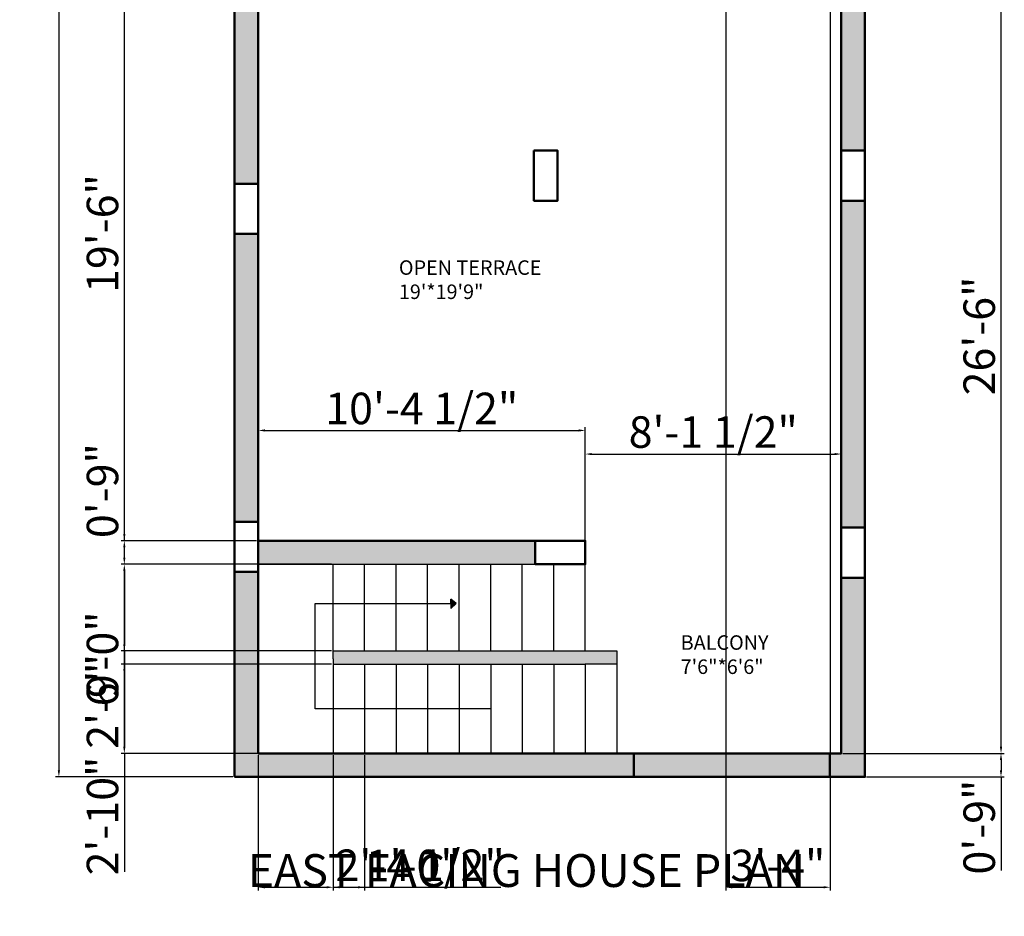
# Model space of a CAD drawing. Units: inches. Extents: x 2063 to 3370, y 2091 to 2971.
# Tile 11 of 14: x 2986 to 3360, y 2091 to 2433. Entities that reach past the tile are written whole.
import ezdxf

# ---------------------------------------------------------------- set-up
doc = ezdxf.new("R2010")
doc.units = ezdxf.units.IN
for name, color, linetype, lineweight in [('A-ANNO-DIMS', 2, 'Continuous', 18), ('A-ANNO-TEXT', 7, 'Continuous', 18), ('A-AREA-IDEN', 3, 'Continuous', 18), ('A-COLS', 7, 'Continuous', 50), ('A-FLOR-STRS', 3, 'Continuous', 25), ('A-WALL', 7, 'Continuous', 50), ('A-WALL-PATT', 8, 'Continuous', 13)]:
    doc.layers.add(name, color=color, linetype=linetype, lineweight=lineweight)
doc.styles.get("Standard").update_dxf_attribs({"font": 'arial.ttf'})
doc.dimstyles.new('ISO-25', dxfattribs={"dimtxt": 12, "dimasz": 2.5, "dimexe": 1.25, "dimexo": 0.625, "dimtad": 1, "dimdec": 0, "dimlunit": 4, "dimtxsty": 'Standard', "dimcen": 2.5, "dimadec": 0, "dimazin": 0, "dimtfac": 1, "dimtdec": 0, "dimtmove": 0, "dimatfit": 3, "dimfxl": 1, "dimarcsym": 0})

# ---------------------------------------------------------------- blocks, each defined once
blk = doc.blocks.new('*D10')
at = {"layer": 'A-ANNO-DIMS', "color": 0, "lineweight": -2, "transparency": 16777216}
for p, q in [((3066.79, 2864.43), (2999.25, 2864.43)), ((3000.5, 2861.93), (3000.5, 2146.93)), ((3066.79, 2144.43), (2999.25, 2144.43))]:
    blk.add_line(p, q, dxfattribs=at)
at = {"layer": 'A-ANNO-DIMS', "color": 0, "transparency": 16777216}
for points in [[(3000.09, 2861.93), (3000.92, 2861.93), (3000.5, 2864.43)], [(3000.09, 2146.93), (3000.92, 2146.93), (3000.5, 2144.43)]]:
    blk.add_solid(points, dxfattribs=at)
at = {"layer": 'Defpoints', "color": 0, "transparency": 16777216}
for p in [(3067.42, 2864.43), (3000.5, 2144.43), (3067.42, 2144.43)]:
    blk.add_point(p, dxfattribs=at)
at = {"layer": 'A-ANNO-DIMS', "color": 0, "transparency": 16777216, "insert": (2993.75, 2504.43), "char_height": 12, "attachment_point": 5, "rotation": 90}
blk.add_mtext("60'", dxfattribs=at)
blk = doc.blocks.new('*D144')
at = {"layer": 'A-ANNO-DIMS', "color": 0, "lineweight": -2, "transparency": 16777216}
for p, q in [((3076.42, 2152.8), (3076.42, 2101.18)), ((3104.92, 2152.8), (3104.92, 2101.18)), ((3078.92, 2102.43), (3102.42, 2102.43)), ((3104.92, 2102.43), (3168.73, 2102.43))]:
    blk.add_line(p, q, dxfattribs=at)
at = {"layer": 'A-ANNO-DIMS', "color": 0, "transparency": 16777216}
for points in [[(3078.92, 2102.84), (3078.92, 2102.01), (3076.42, 2102.43)], [(3102.42, 2102.84), (3102.42, 2102.01), (3104.92, 2102.43)]]:
    blk.add_solid(points, dxfattribs=at)
at = {"layer": 'Defpoints', "color": 0, "transparency": 16777216}
for p in [(3076.42, 2153.43), (3104.92, 2153.43), (3104.92, 2102.43)]:
    blk.add_point(p, dxfattribs=at)
at = {"layer": 'A-ANNO-DIMS', "color": 0, "transparency": 16777216, "insert": (3138.07, 2109.26), "char_height": 12, "attachment_point": 5}
blk.add_mtext('2\'-4 1/2"', dxfattribs=at)
blk = doc.blocks.new('*D145')
at = {"layer": 'A-ANNO-DIMS', "color": 0, "lineweight": -2, "transparency": 16777216}
for p, q in [((3104.92, 2152.8), (3104.92, 2101.18)), ((3116.92, 2152.8), (3116.92, 2101.18)), ((3107.42, 2102.43), (3114.42, 2102.43)), ((3116.92, 2102.43), (3151.44, 2102.43))]:
    blk.add_line(p, q, dxfattribs=at)
at = {"layer": 'A-ANNO-DIMS', "color": 0, "transparency": 16777216}
for points in [[(3107.42, 2102.84), (3107.42, 2102.01), (3104.92, 2102.43)], [(3114.42, 2102.84), (3114.42, 2102.01), (3116.92, 2102.43)]]:
    blk.add_solid(points, dxfattribs=at)
at = {"layer": 'Defpoints', "color": 0, "transparency": 16777216}
for p in [(3104.92, 2153.43), (3116.92, 2153.43), (3116.92, 2102.43)]:
    blk.add_point(p, dxfattribs=at)
at = {"layer": 'A-ANNO-DIMS', "color": 0, "transparency": 16777216, "insert": (3135.43, 2109.18), "char_height": 12, "attachment_point": 5}
blk.add_mtext('1\'-0"', dxfattribs=at)
blk = doc.blocks.new('*D146')
at = {"layer": 'A-ANNO-DIMS', "color": 0, "lineweight": -2, "transparency": 16777216}
for p, q in [((3076.42, 2235.05), (3076.42, 2277.68)), ((3078.92, 2276.43), (3198.42, 2276.43)), ((3200.92, 2235.05), (3200.92, 2277.68))]:
    blk.add_line(p, q, dxfattribs=at)
at = {"layer": 'A-ANNO-DIMS', "color": 0, "transparency": 16777216}
for points in [[(3078.92, 2276.84), (3078.92, 2276.01), (3076.42, 2276.43)], [(3198.42, 2276.84), (3198.42, 2276.01), (3200.92, 2276.43)]]:
    blk.add_solid(points, dxfattribs=at)
at = {"layer": 'Defpoints', "color": 0, "transparency": 16777216}
for p in [(3200.92, 2276.43), (3076.42, 2234.43), (3200.92, 2234.43)]:
    blk.add_point(p, dxfattribs=at)
at = {"layer": 'A-ANNO-DIMS', "color": 0, "transparency": 16777216, "insert": (3138.67, 2283.26), "char_height": 12, "attachment_point": 5}
blk.add_mtext('10\'-4 1/2"', dxfattribs=at)
blk = doc.blocks.new('*D147')
at = {"layer": 'A-ANNO-DIMS', "color": 0, "lineweight": -2, "transparency": 16777216}
for p, q in [((3200.92, 2226.05), (3200.92, 2268.68)), ((3298.42, 2226.05), (3298.42, 2268.68)), ((3203.42, 2267.43), (3295.92, 2267.43))]:
    blk.add_line(p, q, dxfattribs=at)
at = {"layer": 'A-ANNO-DIMS', "color": 0, "transparency": 16777216}
for points in [[(3203.42, 2267.84), (3203.42, 2267.01), (3200.92, 2267.43)], [(3295.92, 2267.84), (3295.92, 2267.01), (3298.42, 2267.43)]]:
    blk.add_solid(points, dxfattribs=at)
at = {"layer": 'Defpoints', "color": 0, "transparency": 16777216}
for p in [(3298.42, 2267.43), (3200.92, 2225.43), (3298.42, 2225.43)]:
    blk.add_point(p, dxfattribs=at)
at = {"layer": 'A-ANNO-DIMS', "color": 0, "transparency": 16777216, "insert": (3249.67, 2274.26), "char_height": 12, "attachment_point": 5}
blk.add_mtext('8\'-1 1/2"', dxfattribs=at)
blk = doc.blocks.new('*D149')
at = {"layer": 'A-ANNO-DIMS', "color": 0, "lineweight": -2, "transparency": 16777216}
for p, q in [((3075.79, 2225.43), (3024.17, 2225.43)), ((3025.42, 2155.93), (3025.42, 2222.93)), ((3075.79, 2153.43), (3024.17, 2153.43))]:
    blk.add_line(p, q, dxfattribs=at)
at = {"layer": 'A-ANNO-DIMS', "color": 0, "transparency": 16777216}
for points in [[(3025, 2222.93), (3025.83, 2222.93), (3025.42, 2225.43)], [(3025, 2155.93), (3025.83, 2155.93), (3025.42, 2153.43)]]:
    blk.add_solid(points, dxfattribs=at)
at = {"layer": 'Defpoints', "color": 0, "transparency": 16777216}
for p in [(3025.42, 2225.43), (3076.42, 2225.43), (3076.42, 2153.43)]:
    blk.add_point(p, dxfattribs=at)
at = {"layer": 'A-ANNO-DIMS', "color": 0, "transparency": 16777216, "insert": (3018.66, 2189.43), "char_height": 12, "attachment_point": 5, "rotation": 90}
blk.add_mtext('6\'-0"', dxfattribs=at)
blk = doc.blocks.new('*D150')
at = {"layer": 'A-ANNO-DIMS', "color": 0, "lineweight": -2, "transparency": 16777216}
for p, q in [((3025.42, 2234.43), (3025.42, 2270.08)), ((3075.79, 2234.43), (3024.17, 2234.43)), ((3025.42, 2227.93), (3025.42, 2231.93)), ((3075.79, 2225.43), (3024.17, 2225.43))]:
    blk.add_line(p, q, dxfattribs=at)
at = {"layer": 'A-ANNO-DIMS', "color": 0, "transparency": 16777216}
for points in [[(3025, 2231.93), (3025.83, 2231.93), (3025.42, 2234.43)], [(3025, 2227.93), (3025.83, 2227.93), (3025.42, 2225.43)]]:
    blk.add_solid(points, dxfattribs=at)
at = {"layer": 'Defpoints', "color": 0, "transparency": 16777216}
for p in [(3025.42, 2234.43), (3076.42, 2234.43), (3076.42, 2225.43)]:
    blk.add_point(p, dxfattribs=at)
at = {"layer": 'A-ANNO-DIMS', "color": 0, "transparency": 16777216, "insert": (3018.66, 2253.5), "char_height": 12, "attachment_point": 5, "rotation": 90}
blk.add_mtext('0\'-9"', dxfattribs=at)
blk = doc.blocks.new('*D151')
at = {"layer": 'A-ANNO-DIMS', "color": 0, "lineweight": -2, "transparency": 16777216}
for p, q in [((3075.79, 2468.43), (3024.17, 2468.43)), ((3025.42, 2236.93), (3025.42, 2465.93)), ((3075.79, 2234.43), (3024.17, 2234.43))]:
    blk.add_line(p, q, dxfattribs=at)
at = {"layer": 'A-ANNO-DIMS', "color": 0, "transparency": 16777216}
for points in [[(3025, 2465.93), (3025.83, 2465.93), (3025.42, 2468.43)], [(3025, 2236.93), (3025.83, 2236.93), (3025.42, 2234.43)]]:
    blk.add_solid(points, dxfattribs=at)
at = {"layer": 'Defpoints', "color": 0, "transparency": 16777216}
for p in [(3025.42, 2468.43), (3076.42, 2468.43), (3076.42, 2234.43)]:
    blk.add_point(p, dxfattribs=at)
at = {"layer": 'A-ANNO-DIMS', "color": 0, "transparency": 16777216, "insert": (3018.66, 2351.43), "char_height": 12, "attachment_point": 5, "rotation": 90}
blk.add_mtext('19\'-6"', dxfattribs=at)
blk = doc.blocks.new('*D160')
at = {"layer": 'A-ANNO-DIMS', "color": 0, "lineweight": -2, "transparency": 16777216}
for p, q in [((3299.04, 2153.43), (3360.49, 2153.43)), ((3359.24, 2150.93), (3359.24, 2146.93)), ((3308.04, 2144.43), (3360.49, 2144.43)), ((3359.24, 2144.43), (3359.24, 2108.78))]:
    blk.add_line(p, q, dxfattribs=at)
at = {"layer": 'A-ANNO-DIMS', "color": 0, "transparency": 16777216}
for points in [[(3358.82, 2150.93), (3359.66, 2150.93), (3359.24, 2153.43)], [(3358.82, 2146.93), (3359.66, 2146.93), (3359.24, 2144.43)]]:
    blk.add_solid(points, dxfattribs=at)
at = {"layer": 'Defpoints', "color": 0, "transparency": 16777216}
for p in [(3298.42, 2153.43), (3307.42, 2144.43), (3359.24, 2144.43)]:
    blk.add_point(p, dxfattribs=at)
at = {"layer": 'A-ANNO-DIMS', "color": 0, "transparency": 16777216, "insert": (3352.49, 2125.35), "char_height": 12, "attachment_point": 5, "rotation": 90}
blk.add_mtext('0\'-9"', dxfattribs=at)
blk = doc.blocks.new('*D161')
at = {"layer": 'A-ANNO-DIMS', "color": 0, "lineweight": -2, "transparency": 16777216}
for p, q in [((3294.79, 2471.41), (3360.49, 2471.41)), ((3359.24, 2155.93), (3359.24, 2468.91)), ((3299.04, 2153.43), (3360.49, 2153.43))]:
    blk.add_line(p, q, dxfattribs=at)
at = {"layer": 'A-ANNO-DIMS', "color": 0, "transparency": 16777216}
for points in [[(3358.82, 2468.91), (3359.66, 2468.91), (3359.24, 2471.41)], [(3358.82, 2155.93), (3359.66, 2155.93), (3359.24, 2153.43)]]:
    blk.add_solid(points, dxfattribs=at)
at = {"layer": 'Defpoints', "color": 0, "transparency": 16777216}
for p in [(3294.16, 2471.41), (3359.24, 2471.41), (3298.42, 2153.43)]:
    blk.add_point(p, dxfattribs=at)
at = {"layer": 'A-ANNO-DIMS', "color": 0, "transparency": 16777216, "insert": (3352.49, 2312.42), "char_height": 12, "attachment_point": 5, "rotation": 90}
blk.add_mtext('26\'-6"', dxfattribs=at)
blk = doc.blocks.new('*D171')
at = {"layer": 'A-ANNO-DIMS', "color": 0, "lineweight": -2, "transparency": 16777216}
for p, q in [((3104.29, 2225.43), (3024.17, 2225.43)), ((3025.42, 2222.93), (3025.42, 2194.93)), ((3104.29, 2192.43), (3024.17, 2192.43)), ((3025.42, 2192.43), (3025.42, 2156.57))]:
    blk.add_line(p, q, dxfattribs=at)
at = {"layer": 'A-ANNO-DIMS', "color": 0, "transparency": 16777216}
for points in [[(3025, 2222.93), (3025.83, 2222.93), (3025.42, 2225.43)], [(3025, 2194.93), (3025.83, 2194.93), (3025.42, 2192.43)]]:
    blk.add_solid(points, dxfattribs=at)
at = {"layer": 'Defpoints', "color": 0, "transparency": 16777216}
for p in [(3104.92, 2225.43), (3025.42, 2192.43), (3104.92, 2192.43)]:
    blk.add_point(p, dxfattribs=at)
at = {"layer": 'A-ANNO-DIMS', "color": 0, "transparency": 16777216, "insert": (3018.66, 2173.25), "char_height": 12, "attachment_point": 5, "rotation": 90}
blk.add_mtext('2\'-9"', dxfattribs=at)
blk = doc.blocks.new('*D172')
at = {"layer": 'A-ANNO-DIMS', "color": 0, "lineweight": -2, "transparency": 16777216}
for p, q in [((3104.29, 2187.43), (3024.17, 2187.43)), ((3025.42, 2184.93), (3025.42, 2155.93)), ((3104.29, 2153.43), (3024.17, 2153.43)), ((3025.42, 2153.43), (3025.42, 2108.25))]:
    blk.add_line(p, q, dxfattribs=at)
at = {"layer": 'A-ANNO-DIMS', "color": 0, "transparency": 16777216}
for points in [[(3025, 2184.93), (3025.83, 2184.93), (3025.42, 2187.43)], [(3025, 2155.93), (3025.83, 2155.93), (3025.42, 2153.43)]]:
    blk.add_solid(points, dxfattribs=at)
at = {"layer": 'Defpoints', "color": 0, "transparency": 16777216}
for p in [(3104.92, 2187.43), (3025.42, 2153.43), (3104.92, 2153.43)]:
    blk.add_point(p, dxfattribs=at)
at = {"layer": 'A-ANNO-DIMS', "color": 0, "transparency": 16777216, "insert": (3018.66, 2129.59), "char_height": 12, "attachment_point": 5, "rotation": 90}
blk.add_mtext('2\'-10"', dxfattribs=at)
blk = doc.blocks.new('*D176')
at = {"layer": 'A-ANNO-DIMS', "color": 0, "lineweight": -2, "transparency": 16777216}
for p, q in [((3254.4, 2476.8), (3254.4, 2101.18)), ((3294.16, 2470.78), (3294.16, 2101.18)), ((3256.9, 2102.43), (3291.66, 2102.43))]:
    blk.add_line(p, q, dxfattribs=at)
at = {"layer": 'A-ANNO-DIMS', "color": 0, "transparency": 16777216}
for points in [[(3256.9, 2102.84), (3256.9, 2102.01), (3254.4, 2102.43)], [(3291.66, 2102.84), (3291.66, 2102.01), (3294.16, 2102.43)]]:
    blk.add_solid(points, dxfattribs=at)
at = {"layer": 'Defpoints', "color": 0, "transparency": 16777216}
for p in [(3254.4, 2477.43), (3294.16, 2471.41), (3294.16, 2102.43)]:
    blk.add_point(p, dxfattribs=at)
at = {"layer": 'A-ANNO-DIMS', "color": 0, "transparency": 16777216, "insert": (3274.28, 2109.18), "char_height": 12, "attachment_point": 5}
blk.add_mtext('3\'-4"', dxfattribs=at)

msp = doc.modelspace()

# ---------------------------------------------------------------- hatches: boundary and pattern name
at = {"layer": 'A-FLOR-STRS'}
h = msp.add_hatch(color=256, dxfattribs=at)
h.dxf.hatch_style = 1
h.paths.add_polyline_path([(3151.76, 2210.45), (3149.68, 2212.18), (3149.68, 2210.45), (3149.68, 2208.56)])
at = {"layer": 'A-WALL-PATT'}
h = msp.add_hatch(color=256, dxfattribs=at)
h.dxf.hatch_style = 1
h.paths.add_polyline_path([(3181.8, 2234.43), (3076.42, 2234.43), (3076.42, 2232.93), (3076.42, 2225.43), (3181.8, 2225.43)])
h.paths.add_polyline_path([(3212.92, 2192.43), (3200.92, 2192.43), (3104.92, 2192.43), (3104.92, 2189.43), (3104.92, 2187.43), (3200.92, 2187.43), (3212.92, 2187.42)], flags=17)
h.paths.add_polyline_path([(3219.45, 2153.43), (3076.42, 2153.43), (3076.42, 2222.57), (3067.42, 2222.57), (3067.42, 2144.43), (3219.45, 2144.43)])
h.paths.add_polyline_path([(3076.42, 2343.93), (3076.42, 2351.28), (3067.42, 2351.28), (3067.42, 2241.68), (3076.42, 2241.68), (3076.42, 2258.43)])
h.paths.add_polyline_path([(3175.73, 2554.94), (3230.21, 2554.94), (3230.21, 2575.54), (3175.73, 2575.54)], flags=9)
h.paths.add_polyline_path([(3085.27, 2530.92), (3121.9, 2530.92), (3121.9, 2551.53), (3085.27, 2551.53)], flags=9)
h.paths.add_polyline_path([(3089.9, 2596.23), (3114.49, 2596.23), (3114.49, 2616.83), (3089.9, 2616.83)], flags=9)
h.paths.add_polyline_path([(3260.79, 2797.55), (3297.86, 2797.55), (3297.86, 2808.94), (3260.79, 2808.94)], flags=9)
h.paths.add_polyline_path([(3113.05, 2696.74), (3189.97, 2696.74), (3189.97, 2717.35), (3113.05, 2717.35)], flags=9)
h.paths.add_polyline_path([(3226.64, 2835.24), (3234.55, 2835.24), (3234.55, 2846.62), (3226.64, 2846.62)], flags=9)
h.paths.add_polyline_path([(3140.56, 2833.68), (3150.6, 2833.68), (3150.6, 2845.06), (3140.56, 2845.06)], flags=9)
h.paths.add_polyline_path([(3193.53, 2795.64), (3230.6, 2795.64), (3230.6, 2807.02), (3193.53, 2807.02)], flags=9)
h.paths.add_polyline_path([(3225.05, 2726.09), (3287.83, 2726.09), (3287.83, 2746.7), (3225.05, 2746.7)], flags=9)
h = msp.add_hatch(color=256, dxfattribs=at)
h.dxf.hatch_style = 1
h.paths.add_polyline_path([(3294.05, 2153.43), (3219.45, 2153.43), (3219.45, 2144.43), (3294.05, 2144.43)])
h.paths.add_polyline_path([(3307.42, 2220.3), (3298.42, 2220.3), (3298.42, 2153.43), (3294.05, 2153.43), (3294.05, 2144.43), (3307.42, 2144.43)])
h.paths.add_polyline_path([(3076.42, 2468.43), (3076.42, 2477.43), (3076.42, 2514.15), (3067.42, 2514.15), (3067.42, 2370.39), (3076.42, 2370.39)])
h.paths.add_polyline_path([(3307.42, 2525.28), (3298.42, 2525.28), (3298.42, 2523.93), (3298.42, 2466.93), (3298.42, 2383.04), (3307.42, 2383.04)])
h.paths.add_polyline_path([(3307.42, 2363.93), (3298.42, 2363.93), (3298.42, 2239.41), (3307.42, 2239.41)])
h.paths.add_polyline_path([(3235.32, 2180.53), (3274.95, 2180.53), (3274.95, 2201.14), (3235.32, 2201.14)], flags=9)
h.paths.add_polyline_path([(3127.74, 2323.36), (3191.84, 2323.36), (3191.84, 2343.96), (3127.74, 2343.96)], flags=9)
h.paths.add_polyline_path([(3175.73, 2554.94), (3230.21, 2554.94), (3230.21, 2575.54), (3175.73, 2575.54)], flags=9)
h.paths.add_polyline_path([(3085.27, 2530.92), (3121.9, 2530.92), (3121.9, 2551.53), (3085.27, 2551.53)], flags=9)
h.paths.add_polyline_path([(3089.9, 2596.23), (3114.49, 2596.23), (3114.49, 2616.83), (3089.9, 2616.83)], flags=9)
h.paths.add_polyline_path([(3260.79, 2797.55), (3297.86, 2797.55), (3297.86, 2808.94), (3260.79, 2808.94)], flags=9)
h.paths.add_polyline_path([(3113.05, 2696.74), (3189.97, 2696.74), (3189.97, 2717.35), (3113.05, 2717.35)], flags=9)
h.paths.add_polyline_path([(3226.64, 2835.24), (3234.55, 2835.24), (3234.55, 2846.62), (3226.64, 2846.62)], flags=9)
h.paths.add_polyline_path([(3140.56, 2833.68), (3150.6, 2833.68), (3150.6, 2845.06), (3140.56, 2845.06)], flags=9)
h.paths.add_polyline_path([(3193.53, 2795.64), (3230.6, 2795.64), (3230.6, 2807.02), (3193.53, 2807.02)], flags=9)
h.paths.add_polyline_path([(3225.05, 2726.09), (3287.83, 2726.09), (3287.83, 2746.7), (3225.05, 2746.7)], flags=9)
h = msp.add_hatch(color=256, dxfattribs=at)
h.dxf.hatch_style = 1
h.paths.add_polyline_path([(3119.94, 2831.43), (3076.42, 2831.43), (3076.42, 2822.43), (3119.94, 2822.43)])
h.paths.add_polyline_path([(3186.73, 2831.43), (3167.94, 2831.43), (3167.94, 2822.43), (3186.73, 2822.43)])
h.paths.add_polyline_path([(3219.33, 2831.43), (3205.84, 2831.43), (3205.84, 2822.43), (3219.33, 2822.43)])
h.paths.add_polyline_path([(3298.42, 2831.43), (3243.76, 2831.43), (3243.76, 2822.43), (3298.42, 2822.43)])
h.paths.add_polyline_path([(3235.32, 2180.53), (3274.95, 2180.53), (3274.95, 2201.14), (3235.32, 2201.14)], flags=9)
h.paths.add_polyline_path([(3127.74, 2323.36), (3191.84, 2323.36), (3191.84, 2343.96), (3127.74, 2343.96)], flags=9)
h.paths.add_polyline_path([(3175.73, 2554.94), (3230.21, 2554.94), (3230.21, 2575.54), (3175.73, 2575.54)], flags=9)
h.paths.add_polyline_path([(3085.27, 2530.92), (3121.9, 2530.92), (3121.9, 2551.53), (3085.27, 2551.53)], flags=9)
h.paths.add_polyline_path([(3089.9, 2596.23), (3114.49, 2596.23), (3114.49, 2616.83), (3089.9, 2616.83)], flags=9)
h.paths.add_polyline_path([(3113.05, 2696.74), (3189.97, 2696.74), (3189.97, 2717.35), (3113.05, 2717.35)], flags=9)
h.paths.add_polyline_path([(3193.53, 2795.64), (3230.6, 2795.64), (3230.6, 2807.02), (3193.53, 2807.02)], flags=9)
h.paths.add_polyline_path([(3225.05, 2726.09), (3287.83, 2726.09), (3287.83, 2746.7), (3225.05, 2746.7)], flags=9)
h = msp.add_hatch(color=256, dxfattribs=at)
h.dxf.hatch_style = 1
h.paths.add_polyline_path([(3254.4, 2477.43), (3145.42, 2477.43), (3145.42, 2579.43), (3145.42, 2589.96), (3142.89, 2589.96), (3140.92, 2589.96), (3140.92, 2583.93), (3131.92, 2583.93), (3076.42, 2583.93), (3076.42, 2579.43), (3136.42, 2579.43), (3140.92, 2579.43), (3140.92, 2477.43), (3076.42, 2477.43), (3076.42, 2468.43), (3193.42, 2468.43), (3254.4, 2468.43), (3254.4, 2471.41)])
h.paths.add_polyline_path([(3235.32, 2180.53), (3274.95, 2180.53), (3274.95, 2201.14), (3235.32, 2201.14)], flags=9)
h.paths.add_polyline_path([(3127.74, 2323.36), (3191.84, 2323.36), (3191.84, 2343.96), (3127.74, 2343.96)], flags=9)
h.paths.add_polyline_path([(3175.73, 2554.94), (3230.21, 2554.94), (3230.21, 2575.54), (3175.73, 2575.54)], flags=25)
h.paths.add_polyline_path([(3089.9, 2596.23), (3114.49, 2596.23), (3114.49, 2616.83), (3089.9, 2616.83)], flags=9)
h.paths.add_polyline_path([(3260.79, 2797.55), (3297.86, 2797.55), (3297.86, 2808.94), (3260.79, 2808.94)], flags=9)
h.paths.add_polyline_path([(3113.05, 2696.74), (3189.97, 2696.74), (3189.97, 2717.35), (3113.05, 2717.35)], flags=9)
h.paths.add_polyline_path([(3193.53, 2795.64), (3230.6, 2795.64), (3230.6, 2807.02), (3193.53, 2807.02)], flags=9)
h.paths.add_polyline_path([(3225.05, 2726.09), (3287.83, 2726.09), (3287.83, 2746.7), (3225.05, 2746.7)], flags=9)

# ---------------------------------------------------------------- linework, layer by layer
at = {"layer": 'A-COLS'}
for points in [[(3181.4, 2383.04), (3190.4, 2383.04), (3190.4, 2363.93), (3181.4, 2363.93)], [(3298.42, 2383.04), (3307.42, 2383.04), (3307.42, 2363.93), (3298.42, 2363.93)], [(3067.42, 2370.39), (3076.42, 2370.39), (3076.42, 2351.28), (3067.42, 2351.28)], [(3067.42, 2241.68), (3076.42, 2241.68), (3076.42, 2222.57), (3067.42, 2222.57)], [(3298.42, 2239.41), (3307.42, 2239.41), (3307.42, 2220.3), (3298.42, 2220.3)], [(3181.8, 2225.43), (3181.8, 2234.43), (3200.92, 2234.43), (3200.92, 2225.43)]]:
    msp.add_lwpolyline(points, close=True, dxfattribs=at)
at = {"layer": 'A-FLOR-STRS'}
for p, q in [((3076.42, 2225.43), (3200.92, 2225.43)), ((3104.92, 2189.43), (3104.92, 2225.43)), ((3116.92, 2192.43), (3116.92, 2225.43)), ((3128.92, 2192.43), (3128.92, 2225.43)), ((3140.92, 2192.43), (3140.92, 2225.43)), ((3152.92, 2192.43), (3152.92, 2225.43)), ((3164.92, 2192.43), (3164.92, 2225.43)), ((3176.92, 2192.43), (3176.92, 2225.43)), ((3188.92, 2192.43), (3188.92, 2225.43)), ((3200.92, 2192.43), (3200.92, 2225.43)), ((3149.68, 2210.45), (3149.68, 2212.18)), ((3151.76, 2210.45), (3149.68, 2212.18)), ((3098.05, 2170.43), (3098.05, 2210.45)), ((3098.05, 2210.45), (3149.68, 2210.45)), ((3149.68, 2210.45), (3149.68, 2208.56)), ((3149.68, 2208.56), (3151.76, 2210.45)), ((3104.92, 2192.43), (3200.92, 2192.43)), ((3212.92, 2191.04), (3212.92, 2153.43)), ((3104.92, 2189.43), (3104.92, 2153.43)), ((3104.92, 2187.43), (3200.92, 2187.43)), ((3116.92, 2187.43), (3116.92, 2153.43)), ((3128.92, 2187.43), (3128.92, 2153.43)), ((3140.92, 2187.43), (3140.92, 2153.43)), ((3152.92, 2187.43), (3152.92, 2153.43)), ((3164.92, 2187.43), (3164.92, 2153.43)), ((3176.92, 2187.43), (3176.92, 2153.43)), ((3188.92, 2187.43), (3188.92, 2153.43)), ((3200.92, 2187.43), (3200.92, 2153.43)), ((3164.92, 2170.43), (3098.05, 2170.43))]:
    msp.add_line(p, q, dxfattribs=at)
msp.add_lwpolyline([(3200.92, 2192.43), (3212.92, 2192.43), (3212.92, 2187.42), (3200.92, 2187.42), (3200.92, 2187.43)], dxfattribs=at)
at = {"layer": 'A-WALL'}
for p, q in [((3076.42, 2241.68), (3076.42, 2477.43)), ((3076.42, 2468.43), (3076.42, 2348.43)), ((3076.42, 2343.93), (3076.42, 2232.93)), ((3076.42, 2234.43), (3076.42, 2258.43)), ((3181.8, 2234.43), (3076.42, 2234.43)), ((3200.92, 2234.43), (3200.92, 2225.43)), ((3219.45, 2144.43), (3219.45, 2153.43)), ((3219.45, 2153.43), (3298.42, 2153.43)), ((3294.05, 2153.43), (3294.05, 2144.43))]:
    msp.add_line(p, q, dxfattribs=at)
msp.add_lwpolyline([(3067.42, 2144.43), (3307.42, 2144.43), (3307.42, 2864.43), (3067.42, 2864.43)], close=True, dxfattribs=at)
for points in [[(3298.42, 2382.93), (3298.42, 2466.93)], [(3298.42, 2234.43), (3298.42, 2378.43)], [(3076.42, 2225.43), (3076.42, 2153.43), (3219.45, 2153.43)], [(3294.05, 2153.43), (3298.42, 2153.43), (3298.42, 2225.43)]]:
    msp.add_lwpolyline(points, dxfattribs=at)

# ---------------------------------------------------------------- texts
at = {"layer": 'A-ANNO-TEXT', "insert": (3072.38, 2115.04), "char_height": 12.498, "attachment_point": 1}
msp.add_mtext_dynamic_manual_height_columns('EAST FACING HOUSE PLAN', width=239.9528, gutter_width=62.49, heights=[33.82], dxfattribs=at)
at = {"layer": 'A-AREA-IDEN', "attachment_point": 1}
for s, insert, char_height in [('OPEN TERRACE\\P19\'*19\'9"', (3129.96, 2341.22), 5.5229), ('BALCONY\\P7\'6"*6\'6"', (3237.26, 2198.4), 5.523)]:
    msp.add_mtext_dynamic_manual_height_columns(s, width=106.0361, gutter_width=27.61, heights=[0], dxfattribs=dict(at, insert=insert, char_height=char_height))

# ---------------------------------------------------------------- dimensions: what is measured, and where the dimension line sits
at = {"layer": 'A-ANNO-DIMS'}
for base, p1, p2, override, picture, middle in [((3000.5, 2144.43), (3067.42, 2864.43), (3067.42, 2144.43), {"dimclrd": 0, "dimclre": 0, "dimclrt": 0}, '*D10', (2993.75, 2504.43)), ((3359.24, 2471.41), (3298.42, 2153.43), (3294.16, 2471.41), {"dimdec": 1, "dimlfac": 1, "dimrnd": 0, "dimzin": 1, "dimdsep": 46, "dimlunit": 4, "dimfrac": 2}, '*D161', (3352.49, 2312.42)), ((3025.42, 2468.43), (3076.42, 2234.43), (3076.42, 2468.43), {"dimdec": 1, "dimlfac": 1, "dimrnd": 0, "dimzin": 1, "dimdsep": 46, "dimlunit": 4, "dimfrac": 2}, '*D151', (3018.66, 2351.43)), ((3025.42, 2234.43), (3076.42, 2225.43), (3076.42, 2234.43), {"dimdec": 1, "dimlfac": 1, "dimrnd": 0, "dimzin": 1, "dimdsep": 46, "dimlunit": 4, "dimfrac": 2}, '*D150', (3018.66, 2253.5)), ((3025.42, 2225.43), (3076.42, 2153.43), (3076.42, 2225.43), {"dimdec": 1, "dimlfac": 1, "dimrnd": 0, "dimzin": 1, "dimdsep": 46, "dimlunit": 4, "dimfrac": 2}, '*D149', (3018.66, 2189.43)), ((3025.42, 2192.43), (3104.92, 2225.43), (3104.92, 2192.43), {"dimdec": 1, "dimlfac": 1, "dimrnd": 0, "dimzin": 1, "dimdsep": 46, "dimlunit": 4, "dimfrac": 2}, '*D171', (3018.66, 2173.25)), ((3025.42, 2153.43), (3104.92, 2187.43), (3104.92, 2153.43), {"dimdec": 1, "dimlfac": 1, "dimrnd": 0, "dimzin": 1, "dimdsep": 46, "dimlunit": 4, "dimfrac": 2}, '*D172', (3018.66, 2129.59)), ((3359.24, 2144.43), (3298.42, 2153.43), (3307.42, 2144.43), {"dimdec": 1, "dimlfac": 1, "dimrnd": 0, "dimzin": 1, "dimdsep": 46, "dimlunit": 4, "dimfrac": 2}, '*D160', (3352.49, 2125.35))]:
    dim = msp.add_linear_dim(base=base, p1=p1, p2=p2, angle=90, dimstyle='ISO-25', override=override, dxfattribs=at)
    dim.commit()
    dim.dimension.update_dxf_attribs({"geometry": picture, "text_midpoint": middle})
for base, p1, p2, picture, middle in [((3294.16, 2102.43), (3254.4, 2477.43), (3294.16, 2471.41), '*D176', (3274.28, 2109.18)), ((3200.92, 2276.43), (3076.42, 2234.43), (3200.92, 2234.43), '*D146', (3138.67, 2283.26)), ((3298.42, 2267.43), (3200.92, 2225.43), (3298.42, 2225.43), '*D147', (3249.67, 2274.26)), ((3104.92, 2102.43), (3076.42, 2153.43), (3104.92, 2153.43), '*D144', (3138.07, 2109.26)), ((3116.92, 2102.43), (3104.92, 2153.43), (3116.92, 2153.43), '*D145', (3135.43, 2109.18))]:
    dim = msp.add_linear_dim(base=base, p1=p1, p2=p2, dimstyle='ISO-25', override={"dimdec": 1, "dimlfac": 1, "dimrnd": 0, "dimzin": 1, "dimdsep": 46, "dimlunit": 4, "dimfrac": 2}, dxfattribs=at)
    dim.commit()
    dim.dimension.update_dxf_attribs({"geometry": picture, "text_midpoint": middle})

doc.saveas('drawing.dxf')
